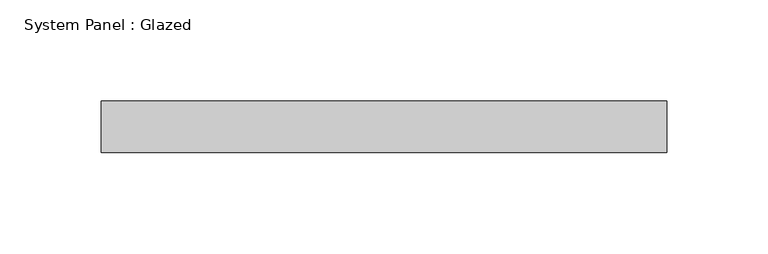
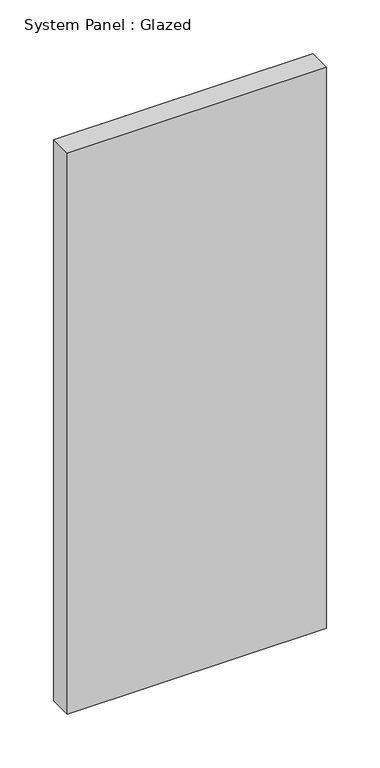
"""IFC4 building model written with IfcOpenShell, lengths in millimetres: plate geometry, System Panel : Glazed."""

from ifc_helpers import new_model, si_unit, origin, origin_with_axes, place, context, project, spatial, polyline, outline, extrude, source, transform, mapped, element, save


def system_panel_glazed_df0efb0a(model_context):
    return source(origin(), model_context, "Body", "SweptSolid", [
        extrude(outline(polyline([(139.7, 19.05), (-139.7, 19.05), (-139.7, 44.45), (139.7, 44.45), (139.7, 19.05)])), origin_with_axes(), (0.0, 0.0, 1.0), 638.9995873),
    ])


if __name__ == "__main__":
    model = new_model("IFC4")
    model_context = context("Model", 3, world=origin())
    ifc_project = project(units=[si_unit("LENGTHUNIT", "METRE", prefix="MILLI")], contexts=[model_context])
    site = spatial("IfcSite", under=ifc_project)
    building = spatial("IfcBuilding", under=site)
    placement = place(None, origin())
    system_panel_glazed_shape = system_panel_glazed_df0efb0a(model_context)
    element("IfcPlate", 1, ObjectType="System Panel : Glazed", at=placement, inside=building, context=model_context, shape_type="MappedRepresentation", body=[
        mapped(system_panel_glazed_shape, transform((0.0, 0.0, 0.0), x_axis=(1.0, 0.0, 0.0), y_axis=(0.0, 1.0, 0.0), z_axis=(0.0, 0.0, 1.0))),
    ])
    save(model, "model.ifc")

# Revit data of these elements
# Type "System Panel : Glazed"
#   Construction Type Id = "GSP4R"
#   Analytic Construction = "1/8 in Pilkington single glazing"
#   Visual Light Transmittance = 0.9
#   Solar Heat Gain Coefficient = 0.86
#   Heat Transfer Coefficient (U) = 1.18115 BTU/(h·ft²·°F)
#   Define Thermal Properties by = 1
# Element 1 (IfcPlate, "System Panel : Glazed")
#   Materials on its faces: "Glass"
# Materials
#   "Glass": class "Glass", colour RGB 0 128 192, transparency 0.75, Description = "Soda Lime Glass", Cost = 0
